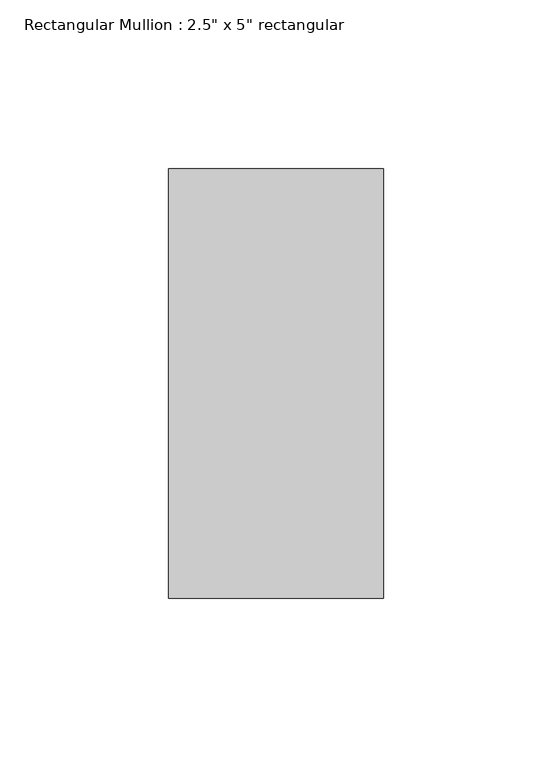
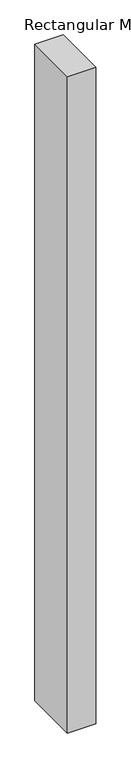
"""IFC4 building model written with IfcOpenShell, lengths in millimetres: member geometry."""

from ifc_helpers import new_model, si_unit, frame, origin, place, context, project, spatial, polyline, outline, extrude, source, transform, mapped, element, save


def member_e29be78d(model_context):
    return source(origin(), model_context, "Body", "SweptSolid", [
        extrude(outline(polyline([(0.0, 63.5), (0.0, -63.5), (-63.5, -63.5), (-63.5, 63.5), (0.0, 63.5)])), frame((0.0, 0.0, -1561.8293392), z_axis=(0.0, 0.0, 1.0), x_axis=(1.0, 0.0, 0.0)), (0.0, 0.0, 1.0), 1561.8293392),
    ])


if __name__ == "__main__":
    model = new_model("IFC4")
    model_context = context("Model", 3, world=origin())
    ifc_project = project(units=[si_unit("LENGTHUNIT", "METRE", prefix="MILLI")], contexts=[model_context])
    site = spatial("IfcSite", under=ifc_project)
    building = spatial("IfcBuilding", under=site)
    placement = place(None, origin())
    member_shape = member_e29be78d(model_context)
    element("IfcMember", 1, ObjectType="Rectangular Mullion : 2.5\" x 5\" rectangular", at=placement, inside=building, context=model_context, shape_type="MappedRepresentation", body=[
        mapped(member_shape, transform((0.0, 0.0, 0.0), x_axis=(1.0, 0.0, 0.0), y_axis=(0.0, 1.0, 0.0), z_axis=(0.0, 0.0, 1.0))),
    ])
    save(model, "model.ifc")

# Revit data of these elements
# Type "Rectangular Mullion : 2.5\" x 5\" rectangular"
#   built-in parameter 1007304 = 0.416667 (stored number, unit not read)
#   built-in parameter 1007301 = 0.104167 (stored number, unit not read)
#   built-in parameter 1007300 = 0.104167 (stored number, unit not read)
# Element 1 (IfcMember, "Rectangular Mullion : 2.5\" x 5\" rectangular")
#   Materials on its faces: "Aluminum"
# Materials
#   "Aluminum": class "Metal", colour RGB 247 247 247, transparency 0, Description = "Aluminum 6061", Cost = 0
